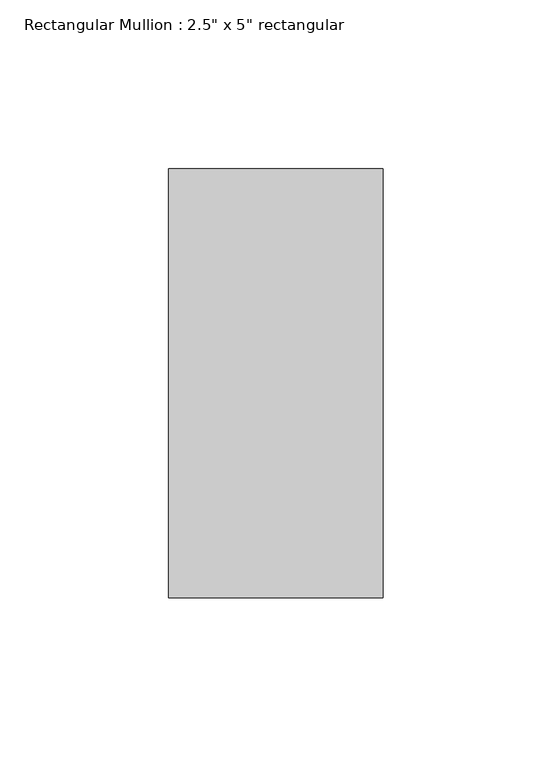
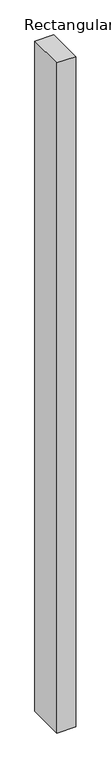
"""IFC4 building model written with IfcOpenShell, lengths in millimetres: member geometry."""

from ifc_helpers import new_model, si_unit, frame, origin, place, context, project, spatial, polyline, outline, extrude, source, transform, mapped, element, save


def member_8cc12096(model_context):
    return source(origin(), model_context, "Body", "SweptSolid", [
        extrude(outline(polyline([(31.75, 63.5), (31.75, -63.5), (-31.75, -63.5), (-31.75, 63.5), (31.75, 63.5)])), frame((0.0, 0.0, -2370.6666667), z_axis=(0.0, 0.0, 1.0), x_axis=(1.0, 0.0, 0.0)), (0.0, 0.0, 1.0), 2370.6666667),
    ])


if __name__ == "__main__":
    model = new_model("IFC4")
    model_context = context("Model", 3, world=origin())
    ifc_project = project(units=[si_unit("LENGTHUNIT", "METRE", prefix="MILLI")], contexts=[model_context])
    site = spatial("IfcSite", under=ifc_project)
    building = spatial("IfcBuilding", under=site)
    placement = place(None, origin())
    member_shape = member_8cc12096(model_context)
    element("IfcMember", 1, ObjectType="Rectangular Mullion : 2.5\" x 5\" rectangular", at=placement, inside=building, context=model_context, shape_type="MappedRepresentation", body=[
        mapped(member_shape, transform((0.0, 0.0, 0.0), x_axis=(1.0, 0.0, 0.0), y_axis=(0.0, 1.0, 0.0), z_axis=(0.0, 0.0, 1.0))),
    ])
    save(model, "model.ifc")

# Revit data of these elements
# Type "Rectangular Mullion : 2.5\" x 5\" rectangular"
#   built-in parameter 1007304 = 0.416667 (stored number, unit not read)
#   built-in parameter 1007301 = 0.104167 (stored number, unit not read)
#   built-in parameter 1007300 = 0.104167 (stored number, unit not read)
# Element 1 (IfcMember, "Rectangular Mullion : 2.5\" x 5\" rectangular")
#   Materials on its faces: "Aluminum"
# Materials
#   "Aluminum": class "Metal", colour RGB 247 247 247, transparency 0, Description = "Aluminum 6061", Cost = 0
